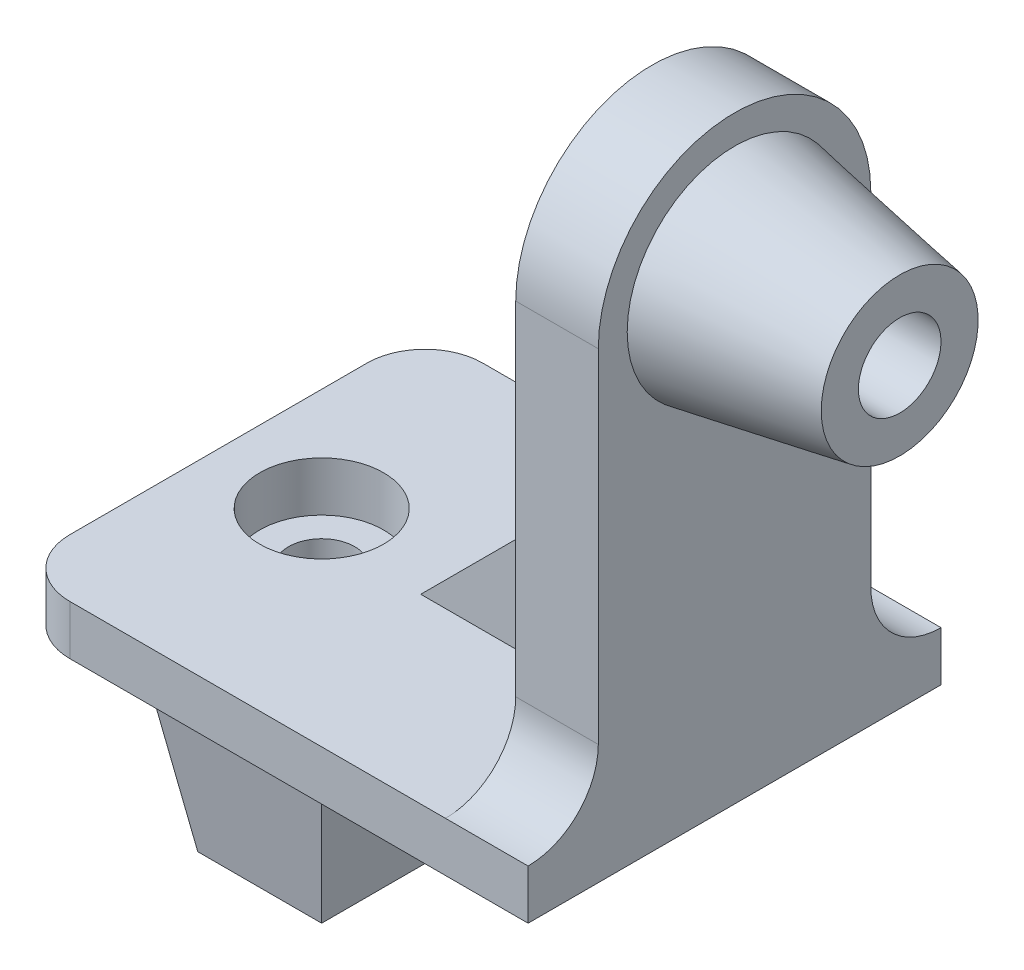
ISO-10303-21;
HEADER;
FILE_DESCRIPTION(('STEP AP214'),'2;1');
FILE_NAME('part.step','',(''),(''),'','','');
FILE_SCHEMA(('AUTOMOTIVE_DESIGN { 1 0 10303 214 1 1 1 1 }'));
ENDSEC;
DATA;
#1=APPLICATION_CONTEXT('core data for automotive mechanical design processes');
#2=APPLICATION_PROTOCOL_DEFINITION('international standard','automotive_design',2000,#1);
#3=PRODUCT_CONTEXT('',#1,'mechanical');
#4=PRODUCT('Part','Part','',(#3));
#5=PRODUCT_RELATED_PRODUCT_CATEGORY('part','',(#4));
#6=PRODUCT_DEFINITION_FORMATION('','',#4);
#7=PRODUCT_DEFINITION_CONTEXT('part definition',#1,'design');
#8=PRODUCT_DEFINITION('design','',#6,#7);
#9=PRODUCT_DEFINITION_SHAPE('','',#8);
#10=(LENGTH_UNIT() NAMED_UNIT(*) SI_UNIT(.MILLI.,.METRE.));
#11=(NAMED_UNIT(*) PLANE_ANGLE_UNIT() SI_UNIT($,.RADIAN.));
#12=(NAMED_UNIT(*) SI_UNIT($,.STERADIAN.) SOLID_ANGLE_UNIT());
#13=UNCERTAINTY_MEASURE_WITH_UNIT(LENGTH_MEASURE(1.E-05),#10,'distance_accuracy_value','');
#14=(GEOMETRIC_REPRESENTATION_CONTEXT(3) GLOBAL_UNCERTAINTY_ASSIGNED_CONTEXT((#13)) GLOBAL_UNIT_ASSIGNED_CONTEXT((#10,
#11,#12)) REPRESENTATION_CONTEXT('',''));
#15=CARTESIAN_POINT('',(0.,0.,0.));
#16=DIRECTION('',(0.,0.,1.));
#17=DIRECTION('',(1.,0.,0.));
#18=AXIS2_PLACEMENT_3D('',#15,#16,#17);
#19=CARTESIAN_POINT('',(-48.5,0.,-36.));
#20=DIRECTION('',(0.,-1.,0.));
#21=DIRECTION('',(0.,0.,-1.));
#22=AXIS2_PLACEMENT_3D('',#19,#20,#21);
#23=PLANE('',#22);
#24=DIRECTION('',(0.,0.,1.));
#25=VECTOR('',#24,1.);
#26=CARTESIAN_POINT('',(-12.5,0.,-25.));
#27=LINE('',#26,#25);
#28=CARTESIAN_POINT('',(-12.5,0.,-25.));
#29=VERTEX_POINT('',#28);
#30=CARTESIAN_POINT('',(-12.5,0.,25.));
#31=VERTEX_POINT('',#30);
#32=EDGE_CURVE('E178',#29,#31,#27,.T.);
#33=ORIENTED_EDGE('',*,*,#32,.F.);
#34=DIRECTION('',(1.,0.,0.));
#35=VECTOR('',#34,1.);
#36=CARTESIAN_POINT('',(-62.5,0.,-25.));
#37=LINE('',#36,#35);
#38=CARTESIAN_POINT('',(-62.5,0.,-25.));
#39=VERTEX_POINT('',#38);
#40=EDGE_CURVE('E257',#39,#29,#37,.T.);
#41=ORIENTED_EDGE('',*,*,#40,.F.);
#42=DIRECTION('',(0.,0.,1.));
#43=VECTOR('',#42,1.);
#44=CARTESIAN_POINT('',(-62.5,0.,36.));
#45=LINE('',#44,#43);
#46=CARTESIAN_POINT('',(-62.5,0.,-36.));
#47=VERTEX_POINT('',#46);
#48=EDGE_CURVE('E339',#47,#39,#45,.T.);
#49=ORIENTED_EDGE('',*,*,#48,.F.);
#50=CARTESIAN_POINT('',(-48.5,0.,-36.));
#51=DIRECTION('',(0.,1.,0.));
#52=DIRECTION('',(0.,0.,-1.));
#53=AXIS2_PLACEMENT_3D('',#50,#51,#52);
#54=CIRCLE('',#53,14.);
#55=CARTESIAN_POINT('',(-48.5,0.,-50.));
#56=VERTEX_POINT('',#55);
#57=EDGE_CURVE('E327',#56,#47,#54,.T.);
#58=ORIENTED_EDGE('',*,*,#57,.F.);
#59=DIRECTION('',(-1.,0.,0.));
#60=VECTOR('',#59,1.);
#61=CARTESIAN_POINT('',(-48.5,0.,-50.));
#62=LINE('',#61,#60);
#63=CARTESIAN_POINT('',(62.5,0.,-50.));
#64=VERTEX_POINT('',#63);
#65=EDGE_CURVE('E326',#64,#56,#62,.T.);
#66=ORIENTED_EDGE('',*,*,#65,.F.);
#67=DIRECTION('',(0.,0.,-1.));
#68=VECTOR('',#67,1.);
#69=CARTESIAN_POINT('',(62.5,0.,50.));
#70=LINE('',#69,#68);
#71=CARTESIAN_POINT('',(62.5,0.,50.));
#72=VERTEX_POINT('',#71);
#73=EDGE_CURVE('E307',#72,#64,#70,.T.);
#74=ORIENTED_EDGE('',*,*,#73,.F.);
#75=DIRECTION('',(1.,0.,0.));
#76=VECTOR('',#75,1.);
#77=CARTESIAN_POINT('',(-48.5,0.,50.));
#78=LINE('',#77,#76);
#79=CARTESIAN_POINT('',(-48.5,0.,50.));
#80=VERTEX_POINT('',#79);
#81=EDGE_CURVE('E378',#80,#72,#78,.T.);
#82=ORIENTED_EDGE('',*,*,#81,.F.);
#83=CARTESIAN_POINT('',(-48.5,0.,36.));
#84=DIRECTION('',(0.,1.,0.));
#85=DIRECTION('',(0.,0.,-1.));
#86=AXIS2_PLACEMENT_3D('',#83,#84,#85);
#87=CIRCLE('',#86,14.);
#88=CARTESIAN_POINT('',(-62.5,0.,36.));
#89=VERTEX_POINT('',#88);
#90=EDGE_CURVE('E334',#89,#80,#87,.T.);
#91=ORIENTED_EDGE('',*,*,#90,.F.);
#92=CARTESIAN_POINT('',(-62.5,0.,25.));
#93=VERTEX_POINT('',#92);
#94=EDGE_CURVE('E329',#93,#89,#45,.T.);
#95=ORIENTED_EDGE('',*,*,#94,.F.);
#96=DIRECTION('',(-1.,0.,0.));
#97=VECTOR('',#96,1.);
#98=CARTESIAN_POINT('',(-62.5,0.,25.));
#99=LINE('',#98,#97);
#100=EDGE_CURVE('E766',#31,#93,#99,.T.);
#101=ORIENTED_EDGE('',*,*,#100,.F.);
#102=EDGE_LOOP('',(#33,#41,#49,#58,#66,#74,#82,#91,#95,#101));
#103=FACE_BOUND('',#102,.T.);
#104=ADVANCED_FACE('F47',(#103),#23,.T.);
#105=CARTESIAN_POINT('',(62.5,12.,50.));
#106=DIRECTION('',(-1.,0.,0.));
#107=DIRECTION('',(0.,0.,1.));
#108=AXIS2_PLACEMENT_3D('',#105,#106,#107);
#109=PLANE('',#108);
#110=ORIENTED_EDGE('',*,*,#73,.T.);
#111=DIRECTION('',(0.,-1.,0.));
#112=VECTOR('',#111,1.);
#113=CARTESIAN_POINT('',(62.5,12.,-50.));
#114=LINE('',#113,#112);
#115=CARTESIAN_POINT('',(62.5,12.,-50.));
#116=VERTEX_POINT('',#115);
#117=EDGE_CURVE('E362',#116,#64,#114,.T.);
#118=ORIENTED_EDGE('',*,*,#117,.F.);
#119=CARTESIAN_POINT('',(62.5,29.,-50.));
#120=DIRECTION('',(-1.,0.,0.));
#121=DIRECTION('',(0.,0.,1.));
#122=AXIS2_PLACEMENT_3D('',#119,#120,#121);
#123=CIRCLE('',#122,17.);
#124=CARTESIAN_POINT('',(62.5,29.,-33.));
#125=VERTEX_POINT('',#124);
#126=EDGE_CURVE('E351',#116,#125,#123,.T.);
#127=ORIENTED_EDGE('',*,*,#126,.T.);
#128=DIRECTION('',(0.,1.,0.));
#129=VECTOR('',#128,1.);
#130=CARTESIAN_POINT('',(62.5,112.,-33.));
#131=LINE('',#130,#129);
#132=CARTESIAN_POINT('',(62.5,112.,-33.));
#133=VERTEX_POINT('',#132);
#134=EDGE_CURVE('E284',#125,#133,#131,.T.);
#135=ORIENTED_EDGE('',*,*,#134,.T.);
#136=CARTESIAN_POINT('',(62.5,112.,0.));
#137=DIRECTION('',(1.,0.,0.));
#138=DIRECTION('',(0.,0.,1.));
#139=AXIS2_PLACEMENT_3D('',#136,#137,#138);
#140=CIRCLE('',#139,33.);
#141=CARTESIAN_POINT('',(62.5,112.,33.));
#142=VERTEX_POINT('',#141);
#143=EDGE_CURVE('E299',#133,#142,#140,.T.);
#144=ORIENTED_EDGE('',*,*,#143,.T.);
#145=DIRECTION('',(0.,-1.,0.));
#146=VECTOR('',#145,1.);
#147=CARTESIAN_POINT('',(62.5,12.,33.));
#148=LINE('',#147,#146);
#149=CARTESIAN_POINT('',(62.5,29.,33.));
#150=VERTEX_POINT('',#149);
#151=EDGE_CURVE('E305',#142,#150,#148,.T.);
#152=ORIENTED_EDGE('',*,*,#151,.T.);
#153=CARTESIAN_POINT('',(62.5,29.,50.));
#154=DIRECTION('',(-1.,0.,0.));
#155=DIRECTION('',(0.,0.,1.));
#156=AXIS2_PLACEMENT_3D('',#153,#154,#155);
#157=CIRCLE('',#156,17.);
#158=CARTESIAN_POINT('',(62.5,12.,50.));
#159=VERTEX_POINT('',#158);
#160=EDGE_CURVE('E348',#150,#159,#157,.T.);
#161=ORIENTED_EDGE('',*,*,#160,.T.);
#162=DIRECTION('',(0.,-1.,0.));
#163=VECTOR('',#162,1.);
#164=CARTESIAN_POINT('',(62.5,12.,50.));
#165=LINE('',#164,#163);
#166=EDGE_CURVE('E322',#159,#72,#165,.T.);
#167=ORIENTED_EDGE('',*,*,#166,.T.);
#168=EDGE_LOOP('',(#110,#118,#127,#135,#144,#152,#161,#167));
#169=FACE_BOUND('',#168,.T.);
#170=CARTESIAN_POINT('',(62.5,112.,0.));
#171=DIRECTION('',(-1.,0.,0.));
#172=DIRECTION('',(0.,0.,1.));
#173=AXIS2_PLACEMENT_3D('',#170,#171,#172);
#174=CIRCLE('',#173,26.);
#175=CARTESIAN_POINT('',(62.5,112.,26.));
#176=VERTEX_POINT('',#175);
#177=EDGE_CURVE('E12',#176,#176,#174,.F.);
#178=ORIENTED_EDGE('',*,*,#177,.F.);
#179=EDGE_LOOP('',(#178));
#180=FACE_BOUND('',#179,.T.);
#181=ADVANCED_FACE('F399',(#169,#180),#109,.F.);
#182=CARTESIAN_POINT('',(-48.5,12.,-36.));
#183=DIRECTION('',(0.,-1.,0.));
#184=DIRECTION('',(0.,0.,-1.));
#185=AXIS2_PLACEMENT_3D('',#182,#183,#184);
#186=PLANE('',#185);
#187=CARTESIAN_POINT('',(-37.5,12.,0.));
#188=DIRECTION('',(0.,1.,0.));
#189=DIRECTION('',(0.,0.,1.));
#190=AXIS2_PLACEMENT_3D('',#187,#188,#189);
#191=CIRCLE('',#190,15.);
#192=CARTESIAN_POINT('',(-37.5,12.,15.));
#193=VERTEX_POINT('',#192);
#194=EDGE_CURVE('E702',#193,#193,#191,.T.);
#195=ORIENTED_EDGE('',*,*,#194,.F.);
#196=EDGE_LOOP('',(#195));
#197=FACE_BOUND('',#196,.T.);
#198=DIRECTION('',(0.,0.,-1.));
#199=VECTOR('',#198,1.);
#200=CARTESIAN_POINT('',(42.5,12.,-33.));
#201=LINE('',#200,#199);
#202=CARTESIAN_POINT('',(42.5,12.,50.));
#203=VERTEX_POINT('',#202);
#204=CARTESIAN_POINT('',(42.5,12.,6.));
#205=VERTEX_POINT('',#204);
#206=EDGE_CURVE('E281',#203,#205,#201,.T.);
#207=ORIENTED_EDGE('',*,*,#206,.T.);
#208=DIRECTION('',(-1.,0.,0.));
#209=VECTOR('',#208,1.);
#210=CARTESIAN_POINT('',(-48.5,12.,6.));
#211=LINE('',#210,#209);
#212=CARTESIAN_POINT('',(-7.49999999999999,12.,6.));
#213=VERTEX_POINT('',#212);
#214=EDGE_CURVE('E279',#205,#213,#211,.T.);
#215=ORIENTED_EDGE('',*,*,#214,.T.);
#216=DIRECTION('',(0.,0.,1.));
#217=VECTOR('',#216,1.);
#218=CARTESIAN_POINT('',(-7.49999999999999,12.,-36.));
#219=LINE('',#218,#217);
#220=CARTESIAN_POINT('',(-7.49999999999999,12.,-6.));
#221=VERTEX_POINT('',#220);
#222=EDGE_CURVE('E282',#213,#221,#219,.F.);
#223=ORIENTED_EDGE('',*,*,#222,.T.);
#224=DIRECTION('',(-1.,0.,0.));
#225=VECTOR('',#224,1.);
#226=CARTESIAN_POINT('',(-48.5,12.,-6.));
#227=LINE('',#226,#225);
#228=CARTESIAN_POINT('',(42.5,12.,-6.));
#229=VERTEX_POINT('',#228);
#230=EDGE_CURVE('E274',#229,#221,#227,.T.);
#231=ORIENTED_EDGE('',*,*,#230,.F.);
#232=CARTESIAN_POINT('',(42.5,12.,-50.));
#233=VERTEX_POINT('',#232);
#234=EDGE_CURVE('E286',#229,#233,#201,.T.);
#235=ORIENTED_EDGE('',*,*,#234,.T.);
#236=DIRECTION('',(-1.,0.,0.));
#237=VECTOR('',#236,1.);
#238=CARTESIAN_POINT('',(-48.5,12.,-50.));
#239=LINE('',#238,#237);
#240=CARTESIAN_POINT('',(-48.5,12.,-50.));
#241=VERTEX_POINT('',#240);
#242=EDGE_CURVE('E314',#233,#241,#239,.T.);
#243=ORIENTED_EDGE('',*,*,#242,.T.);
#244=CARTESIAN_POINT('',(-48.5,12.,-36.));
#245=DIRECTION('',(0.,1.,0.));
#246=DIRECTION('',(0.,0.,-1.));
#247=AXIS2_PLACEMENT_3D('',#244,#245,#246);
#248=CIRCLE('',#247,14.);
#249=CARTESIAN_POINT('',(-62.5,12.,-36.));
#250=VERTEX_POINT('',#249);
#251=EDGE_CURVE('E311',#241,#250,#248,.T.);
#252=ORIENTED_EDGE('',*,*,#251,.T.);
#253=DIRECTION('',(0.,0.,1.));
#254=VECTOR('',#253,1.);
#255=CARTESIAN_POINT('',(-62.5,12.,36.));
#256=LINE('',#255,#254);
#257=CARTESIAN_POINT('',(-62.5,12.,36.));
#258=VERTEX_POINT('',#257);
#259=EDGE_CURVE('E316',#250,#258,#256,.T.);
#260=ORIENTED_EDGE('',*,*,#259,.T.);
#261=CARTESIAN_POINT('',(-48.5,12.,36.));
#262=DIRECTION('',(0.,1.,0.));
#263=DIRECTION('',(0.,0.,-1.));
#264=AXIS2_PLACEMENT_3D('',#261,#262,#263);
#265=CIRCLE('',#264,14.);
#266=CARTESIAN_POINT('',(-48.5,12.,50.));
#267=VERTEX_POINT('',#266);
#268=EDGE_CURVE('E318',#258,#267,#265,.T.);
#269=ORIENTED_EDGE('',*,*,#268,.T.);
#270=DIRECTION('',(1.,0.,0.));
#271=VECTOR('',#270,1.);
#272=CARTESIAN_POINT('',(-48.5,12.,50.));
#273=LINE('',#272,#271);
#274=EDGE_CURVE('E321',#267,#203,#273,.T.);
#275=ORIENTED_EDGE('',*,*,#274,.T.);
#276=EDGE_LOOP('',(#207,#215,#223,#231,#235,#243,#252,#260,#269,#275));
#277=FACE_BOUND('',#276,.T.);
#278=ADVANCED_FACE('F429',(#197,#277),#186,.F.);
#279=CARTESIAN_POINT('',(-48.5,12.,-50.));
#280=DIRECTION('',(0.,0.,1.));
#281=DIRECTION('',(1.,0.,0.));
#282=AXIS2_PLACEMENT_3D('',#279,#280,#281);
#283=PLANE('',#282);
#284=ORIENTED_EDGE('',*,*,#65,.T.);
#285=DIRECTION('',(0.,-1.,0.));
#286=VECTOR('',#285,1.);
#287=CARTESIAN_POINT('',(-48.5,12.,-50.));
#288=LINE('',#287,#286);
#289=EDGE_CURVE('E364',#241,#56,#288,.T.);
#290=ORIENTED_EDGE('',*,*,#289,.F.);
#291=ORIENTED_EDGE('',*,*,#242,.F.);
#292=EDGE_CURVE('E309',#116,#233,#239,.T.);
#293=ORIENTED_EDGE('',*,*,#292,.F.);
#294=ORIENTED_EDGE('',*,*,#117,.T.);
#295=EDGE_LOOP('',(#284,#290,#291,#293,#294));
#296=FACE_BOUND('',#295,.T.);
#297=ADVANCED_FACE('F426',(#296),#283,.F.);
#298=CARTESIAN_POINT('',(-48.5,12.,-36.));
#299=DIRECTION('',(0.,-1.,0.));
#300=DIRECTION('',(0.,0.,-1.));
#301=AXIS2_PLACEMENT_3D('',#298,#299,#300);
#302=CYLINDRICAL_SURFACE('',#301,14.);
#303=ORIENTED_EDGE('',*,*,#57,.T.);
#304=DIRECTION('',(0.,-1.,0.));
#305=VECTOR('',#304,1.);
#306=CARTESIAN_POINT('',(-62.5,12.,-36.));
#307=LINE('',#306,#305);
#308=EDGE_CURVE('E366',#250,#47,#307,.T.);
#309=ORIENTED_EDGE('',*,*,#308,.F.);
#310=ORIENTED_EDGE('',*,*,#251,.F.);
#311=ORIENTED_EDGE('',*,*,#289,.T.);
#312=EDGE_LOOP('',(#303,#309,#310,#311));
#313=FACE_BOUND('',#312,.T.);
#314=ADVANCED_FACE('F470',(#313),#302,.T.);
#315=CARTESIAN_POINT('',(-62.5,12.,36.));
#316=DIRECTION('',(1.,0.,0.));
#317=DIRECTION('',(0.,0.,-1.));
#318=AXIS2_PLACEMENT_3D('',#315,#316,#317);
#319=PLANE('',#318);
#320=ORIENTED_EDGE('',*,*,#48,.T.);
#321=DIRECTION('',(0.,0.,-1.));
#322=VECTOR('',#321,1.);
#323=CARTESIAN_POINT('',(-62.5,0.,-25.));
#324=LINE('',#323,#322);
#325=EDGE_CURVE('E759',#93,#39,#324,.T.);
#326=ORIENTED_EDGE('',*,*,#325,.F.);
#327=ORIENTED_EDGE('',*,*,#94,.T.);
#328=DIRECTION('',(0.,-1.,0.));
#329=VECTOR('',#328,1.);
#330=CARTESIAN_POINT('',(-62.5,12.,36.));
#331=LINE('',#330,#329);
#332=EDGE_CURVE('E371',#258,#89,#331,.T.);
#333=ORIENTED_EDGE('',*,*,#332,.F.);
#334=ORIENTED_EDGE('',*,*,#259,.F.);
#335=ORIENTED_EDGE('',*,*,#308,.T.);
#336=EDGE_LOOP('',(#320,#326,#327,#333,#334,#335));
#337=FACE_BOUND('',#336,.T.);
#338=ADVANCED_FACE('F461',(#337),#319,.F.);
#339=CARTESIAN_POINT('',(-48.5,12.,36.));
#340=DIRECTION('',(0.,-1.,0.));
#341=DIRECTION('',(0.,0.,-1.));
#342=AXIS2_PLACEMENT_3D('',#339,#340,#341);
#343=CYLINDRICAL_SURFACE('',#342,14.);
#344=ORIENTED_EDGE('',*,*,#90,.T.);
#345=DIRECTION('',(0.,-1.,0.));
#346=VECTOR('',#345,1.);
#347=CARTESIAN_POINT('',(-48.5,12.,50.));
#348=LINE('',#347,#346);
#349=EDGE_CURVE('E372',#267,#80,#348,.T.);
#350=ORIENTED_EDGE('',*,*,#349,.F.);
#351=ORIENTED_EDGE('',*,*,#268,.F.);
#352=ORIENTED_EDGE('',*,*,#332,.T.);
#353=EDGE_LOOP('',(#344,#350,#351,#352));
#354=FACE_BOUND('',#353,.T.);
#355=ADVANCED_FACE('F384',(#354),#343,.T.);
#356=CARTESIAN_POINT('',(-48.5,12.,50.));
#357=DIRECTION('',(0.,0.,-1.));
#358=DIRECTION('',(-1.,0.,0.));
#359=AXIS2_PLACEMENT_3D('',#356,#357,#358);
#360=PLANE('',#359);
#361=ORIENTED_EDGE('',*,*,#81,.T.);
#362=ORIENTED_EDGE('',*,*,#166,.F.);
#363=EDGE_CURVE('E319',#203,#159,#273,.T.);
#364=ORIENTED_EDGE('',*,*,#363,.F.);
#365=ORIENTED_EDGE('',*,*,#274,.F.);
#366=ORIENTED_EDGE('',*,*,#349,.T.);
#367=EDGE_LOOP('',(#361,#362,#364,#365,#366));
#368=FACE_BOUND('',#367,.T.);
#369=ADVANCED_FACE('F392',(#368),#360,.F.);
#370=CARTESIAN_POINT('',(42.5,12.,33.));
#371=DIRECTION('',(0.,0.,1.));
#372=DIRECTION('',(0.,-1.,0.));
#373=AXIS2_PLACEMENT_3D('',#370,#371,#372);
#374=PLANE('',#373);
#375=DIRECTION('',(0.,-1.,0.));
#376=VECTOR('',#375,1.);
#377=CARTESIAN_POINT('',(42.5,12.,33.));
#378=LINE('',#377,#376);
#379=CARTESIAN_POINT('',(42.5,112.,33.));
#380=VERTEX_POINT('',#379);
#381=CARTESIAN_POINT('',(42.5,29.,33.));
#382=VERTEX_POINT('',#381);
#383=EDGE_CURVE('E294',#380,#382,#378,.T.);
#384=ORIENTED_EDGE('',*,*,#383,.T.);
#385=DIRECTION('',(1.,0.,0.));
#386=VECTOR('',#385,1.);
#387=CARTESIAN_POINT('',(42.5,29.,33.));
#388=LINE('',#387,#386);
#389=EDGE_CURVE('E360',#382,#150,#388,.T.);
#390=ORIENTED_EDGE('',*,*,#389,.T.);
#391=ORIENTED_EDGE('',*,*,#151,.F.);
#392=DIRECTION('',(1.,0.,0.));
#393=VECTOR('',#392,1.);
#394=CARTESIAN_POINT('',(42.5,112.,33.));
#395=LINE('',#394,#393);
#396=EDGE_CURVE('E303',#380,#142,#395,.T.);
#397=ORIENTED_EDGE('',*,*,#396,.F.);
#398=EDGE_LOOP('',(#384,#390,#391,#397));
#399=FACE_BOUND('',#398,.T.);
#400=ADVANCED_FACE('F406',(#399),#374,.T.);
#401=CARTESIAN_POINT('',(42.5,112.,0.));
#402=DIRECTION('',(1.,0.,0.));
#403=DIRECTION('',(0.,0.,-1.));
#404=AXIS2_PLACEMENT_3D('',#401,#402,#403);
#405=CYLINDRICAL_SURFACE('',#404,33.);
#406=ORIENTED_EDGE('',*,*,#143,.F.);
#407=DIRECTION('',(1.,0.,0.));
#408=VECTOR('',#407,1.);
#409=CARTESIAN_POINT('',(42.5,112.,-33.));
#410=LINE('',#409,#408);
#411=CARTESIAN_POINT('',(42.5,112.,-33.));
#412=VERTEX_POINT('',#411);
#413=EDGE_CURVE('E300',#412,#133,#410,.T.);
#414=ORIENTED_EDGE('',*,*,#413,.F.);
#415=CARTESIAN_POINT('',(42.5,112.,0.));
#416=DIRECTION('',(1.,0.,0.));
#417=DIRECTION('',(0.,0.,1.));
#418=AXIS2_PLACEMENT_3D('',#415,#416,#417);
#419=CIRCLE('',#418,33.);
#420=EDGE_CURVE('E292',#412,#380,#419,.T.);
#421=ORIENTED_EDGE('',*,*,#420,.T.);
#422=ORIENTED_EDGE('',*,*,#396,.T.);
#423=EDGE_LOOP('',(#406,#414,#421,#422));
#424=FACE_BOUND('',#423,.T.);
#425=ADVANCED_FACE('F413',(#424),#405,.T.);
#426=CARTESIAN_POINT('',(42.5,112.,-33.));
#427=DIRECTION('',(0.,0.,-1.));
#428=DIRECTION('',(0.,1.,0.));
#429=AXIS2_PLACEMENT_3D('',#426,#427,#428);
#430=PLANE('',#429);
#431=ORIENTED_EDGE('',*,*,#134,.F.);
#432=DIRECTION('',(1.,0.,0.));
#433=VECTOR('',#432,1.);
#434=CARTESIAN_POINT('',(42.5,29.,-33.));
#435=LINE('',#434,#433);
#436=CARTESIAN_POINT('',(42.5,29.,-33.));
#437=VERTEX_POINT('',#436);
#438=EDGE_CURVE('E358',#125,#437,#435,.F.);
#439=ORIENTED_EDGE('',*,*,#438,.T.);
#440=DIRECTION('',(0.,1.,0.));
#441=VECTOR('',#440,1.);
#442=CARTESIAN_POINT('',(42.5,112.,-33.));
#443=LINE('',#442,#441);
#444=EDGE_CURVE('E289',#437,#412,#443,.T.);
#445=ORIENTED_EDGE('',*,*,#444,.T.);
#446=ORIENTED_EDGE('',*,*,#413,.T.);
#447=EDGE_LOOP('',(#431,#439,#445,#446));
#448=FACE_BOUND('',#447,.T.);
#449=ADVANCED_FACE('F479',(#448),#430,.T.);
#450=CARTESIAN_POINT('',(42.5,112.,0.));
#451=DIRECTION('',(-1.,0.,0.));
#452=DIRECTION('',(0.,0.,1.));
#453=AXIS2_PLACEMENT_3D('',#450,#451,#452);
#454=PLANE('',#453);
#455=CARTESIAN_POINT('',(42.5,112.,0.));
#456=DIRECTION('',(-1.,0.,0.));
#457=DIRECTION('',(0.,0.,1.));
#458=AXIS2_PLACEMENT_3D('',#455,#456,#457);
#459=CIRCLE('',#458,15.);
#460=CARTESIAN_POINT('',(42.5,112.,15.));
#461=VERTEX_POINT('',#460);
#462=EDGE_CURVE('E259',#461,#461,#459,.T.);
#463=ORIENTED_EDGE('',*,*,#462,.F.);
#464=EDGE_LOOP('',(#463));
#465=FACE_BOUND('',#464,.T.);
#466=DIRECTION('',(0.,1.,0.));
#467=VECTOR('',#466,1.);
#468=CARTESIAN_POINT('',(42.5,112.,6.));
#469=LINE('',#468,#467);
#470=CARTESIAN_POINT('',(42.5,62.,6.));
#471=VERTEX_POINT('',#470);
#472=EDGE_CURVE('E59',#205,#471,#469,.T.);
#473=ORIENTED_EDGE('',*,*,#472,.F.);
#474=ORIENTED_EDGE('',*,*,#206,.F.);
#475=CARTESIAN_POINT('',(42.5,29.,50.));
#476=DIRECTION('',(-1.,0.,0.));
#477=DIRECTION('',(0.,0.,1.));
#478=AXIS2_PLACEMENT_3D('',#475,#476,#477);
#479=CIRCLE('',#478,17.);
#480=EDGE_CURVE('E346',#203,#382,#479,.F.);
#481=ORIENTED_EDGE('',*,*,#480,.T.);
#482=ORIENTED_EDGE('',*,*,#383,.F.);
#483=ORIENTED_EDGE('',*,*,#420,.F.);
#484=ORIENTED_EDGE('',*,*,#444,.F.);
#485=CARTESIAN_POINT('',(42.5,29.,-50.));
#486=DIRECTION('',(-1.,0.,0.));
#487=DIRECTION('',(0.,0.,1.));
#488=AXIS2_PLACEMENT_3D('',#485,#486,#487);
#489=CIRCLE('',#488,17.);
#490=EDGE_CURVE('E355',#437,#233,#489,.F.);
#491=ORIENTED_EDGE('',*,*,#490,.T.);
#492=ORIENTED_EDGE('',*,*,#234,.F.);
#493=DIRECTION('',(0.,1.,0.));
#494=VECTOR('',#493,1.);
#495=CARTESIAN_POINT('',(42.5,112.,-6.));
#496=LINE('',#495,#494);
#497=CARTESIAN_POINT('',(42.5,62.,-6.));
#498=VERTEX_POINT('',#497);
#499=EDGE_CURVE('E343',#229,#498,#496,.T.);
#500=ORIENTED_EDGE('',*,*,#499,.T.);
#501=DIRECTION('',(0.,0.,1.));
#502=VECTOR('',#501,1.);
#503=CARTESIAN_POINT('',(42.5,62.,0.));
#504=LINE('',#503,#502);
#505=EDGE_CURVE('E344',#471,#498,#504,.F.);
#506=ORIENTED_EDGE('',*,*,#505,.F.);
#507=EDGE_LOOP('',(#473,#474,#481,#482,#483,#484,#491,#492,#500,#506));
#508=FACE_BOUND('',#507,.T.);
#509=ADVANCED_FACE('F410',(#465,#508),#454,.T.);
#510=CARTESIAN_POINT('',(-48.5,29.,-50.));
#511=DIRECTION('',(1.,0.,0.));
#512=DIRECTION('',(0.,0.,-1.));
#513=AXIS2_PLACEMENT_3D('',#510,#511,#512);
#514=CYLINDRICAL_SURFACE('',#513,17.);
#515=ORIENTED_EDGE('',*,*,#490,.F.);
#516=ORIENTED_EDGE('',*,*,#438,.F.);
#517=ORIENTED_EDGE('',*,*,#126,.F.);
#518=ORIENTED_EDGE('',*,*,#292,.T.);
#519=EDGE_LOOP('',(#515,#516,#517,#518));
#520=FACE_BOUND('',#519,.T.);
#521=ADVANCED_FACE('F421',(#520),#514,.F.);
#522=CARTESIAN_POINT('',(42.5,29.,50.));
#523=DIRECTION('',(1.,0.,0.));
#524=DIRECTION('',(0.,0.,-1.));
#525=AXIS2_PLACEMENT_3D('',#522,#523,#524);
#526=CYLINDRICAL_SURFACE('',#525,17.);
#527=ORIENTED_EDGE('',*,*,#480,.F.);
#528=ORIENTED_EDGE('',*,*,#363,.T.);
#529=ORIENTED_EDGE('',*,*,#160,.F.);
#530=ORIENTED_EDGE('',*,*,#389,.F.);
#531=EDGE_LOOP('',(#527,#528,#529,#530));
#532=FACE_BOUND('',#531,.T.);
#533=ADVANCED_FACE('F51',(#532),#526,.F.);
#534=CARTESIAN_POINT('',(-7.49999999999999,12.,0.));
#535=DIRECTION('',(0.707106781186548,-0.707106781186548,0.));
#536=DIRECTION('',(0.707106781186547,0.707106781186547,0.));
#537=AXIS2_PLACEMENT_3D('',#534,#535,#536);
#538=PLANE('',#537);
#539=ORIENTED_EDGE('',*,*,#222,.F.);
#540=DIRECTION('',(0.707106781186547,0.707106781186547,0.));
#541=VECTOR('',#540,1.);
#542=CARTESIAN_POINT('',(-7.49999999999999,12.,6.));
#543=LINE('',#542,#541);
#544=EDGE_CURVE('E275',#213,#471,#543,.T.);
#545=ORIENTED_EDGE('',*,*,#544,.T.);
#546=ORIENTED_EDGE('',*,*,#505,.T.);
#547=DIRECTION('',(0.707106781186547,0.707106781186547,0.));
#548=VECTOR('',#547,1.);
#549=CARTESIAN_POINT('',(-7.49999999999999,12.,-6.));
#550=LINE('',#549,#548);
#551=EDGE_CURVE('E74',#221,#498,#550,.T.);
#552=ORIENTED_EDGE('',*,*,#551,.F.);
#553=EDGE_LOOP('',(#539,#545,#546,#552));
#554=FACE_BOUND('',#553,.T.);
#555=ADVANCED_FACE('F436',(#554),#538,.F.);
#556=CARTESIAN_POINT('',(0.,72.5,6.));
#557=DIRECTION('',(0.,0.,1.));
#558=DIRECTION('',(1.,0.,0.));
#559=AXIS2_PLACEMENT_3D('',#556,#557,#558);
#560=PLANE('',#559);
#561=ORIENTED_EDGE('',*,*,#214,.F.);
#562=ORIENTED_EDGE('',*,*,#472,.T.);
#563=ORIENTED_EDGE('',*,*,#544,.F.);
#564=EDGE_LOOP('',(#561,#562,#563));
#565=FACE_BOUND('',#564,.T.);
#566=ADVANCED_FACE('F438',(#565),#560,.T.);
#567=CARTESIAN_POINT('',(0.,72.5,-6.));
#568=DIRECTION('',(0.,0.,1.));
#569=DIRECTION('',(1.,0.,0.));
#570=AXIS2_PLACEMENT_3D('',#567,#568,#569);
#571=PLANE('',#570);
#572=ORIENTED_EDGE('',*,*,#499,.F.);
#573=ORIENTED_EDGE('',*,*,#230,.T.);
#574=ORIENTED_EDGE('',*,*,#551,.T.);
#575=EDGE_LOOP('',(#572,#573,#574));
#576=FACE_BOUND('',#575,.T.);
#577=ADVANCED_FACE('F432',(#576),#571,.F.);
#578=CARTESIAN_POINT('',(102.5,112.,0.));
#579=DIRECTION('',(-1.,0.,0.));
#580=DIRECTION('',(0.,0.,1.));
#581=AXIS2_PLACEMENT_3D('',#578,#579,#580);
#582=CONICAL_SURFACE('',#581,19.,0.173245666452365);
#583=ORIENTED_EDGE('',*,*,#177,.T.);
#584=EDGE_LOOP('',(#583));
#585=FACE_BOUND('',#584,.T.);
#586=CARTESIAN_POINT('',(102.5,112.,0.));
#587=DIRECTION('',(-1.,0.,0.));
#588=DIRECTION('',(0.,0.,1.));
#589=AXIS2_PLACEMENT_3D('',#586,#587,#588);
#590=CIRCLE('',#589,19.);
#591=CARTESIAN_POINT('',(102.5,112.,19.));
#592=VERTEX_POINT('',#591);
#593=EDGE_CURVE('E267',#592,#592,#590,.T.);
#594=ORIENTED_EDGE('',*,*,#593,.T.);
#595=EDGE_LOOP('',(#594));
#596=FACE_BOUND('',#595,.T.);
#597=ADVANCED_FACE('F447',(#585,#596),#582,.T.);
#598=CARTESIAN_POINT('',(102.5,131.,0.));
#599=DIRECTION('',(-1.,0.,0.));
#600=DIRECTION('',(0.,0.,1.));
#601=AXIS2_PLACEMENT_3D('',#598,#599,#600);
#602=PLANE('',#601);
#603=ORIENTED_EDGE('',*,*,#593,.F.);
#604=EDGE_LOOP('',(#603));
#605=FACE_BOUND('',#604,.T.);
#606=CARTESIAN_POINT('',(102.5,112.,0.));
#607=DIRECTION('',(-1.,0.,0.));
#608=DIRECTION('',(0.,0.,1.));
#609=AXIS2_PLACEMENT_3D('',#606,#607,#608);
#610=CIRCLE('',#609,9.99999999999999);
#611=CARTESIAN_POINT('',(102.5,112.,9.99999999999999));
#612=VERTEX_POINT('',#611);
#613=EDGE_CURVE('E262',#612,#612,#610,.T.);
#614=ORIENTED_EDGE('',*,*,#613,.T.);
#615=EDGE_LOOP('',(#614));
#616=FACE_BOUND('',#615,.T.);
#617=ADVANCED_FACE('F563',(#605,#616),#602,.F.);
#618=CARTESIAN_POINT('',(62.5,112.,0.));
#619=DIRECTION('',(-1.,0.,0.));
#620=DIRECTION('',(0.,0.,1.));
#621=AXIS2_PLACEMENT_3D('',#618,#619,#620);
#622=CYLINDRICAL_SURFACE('',#621,9.99999999999999);
#623=ORIENTED_EDGE('',*,*,#613,.F.);
#624=EDGE_LOOP('',(#623));
#625=FACE_BOUND('',#624,.T.);
#626=CARTESIAN_POINT('',(54.5,112.,0.));
#627=DIRECTION('',(-1.,0.,0.));
#628=DIRECTION('',(0.,0.,1.));
#629=AXIS2_PLACEMENT_3D('',#626,#627,#628);
#630=CIRCLE('',#629,10.);
#631=CARTESIAN_POINT('',(54.5,112.,10.));
#632=VERTEX_POINT('',#631);
#633=EDGE_CURVE('E253',#632,#632,#630,.T.);
#634=ORIENTED_EDGE('',*,*,#633,.T.);
#635=EDGE_LOOP('',(#634));
#636=FACE_BOUND('',#635,.T.);
#637=ADVANCED_FACE('F573',(#625,#636),#622,.F.);
#638=CARTESIAN_POINT('',(54.5,112.,0.));
#639=DIRECTION('',(-1.,0.,0.));
#640=DIRECTION('',(0.,0.,1.));
#641=AXIS2_PLACEMENT_3D('',#638,#639,#640);
#642=CYLINDRICAL_SURFACE('',#641,15.);
#643=CARTESIAN_POINT('',(54.5,112.,0.));
#644=DIRECTION('',(-1.,0.,0.));
#645=DIRECTION('',(0.,0.,1.));
#646=AXIS2_PLACEMENT_3D('',#643,#644,#645);
#647=CIRCLE('',#646,15.);
#648=CARTESIAN_POINT('',(54.5,112.,15.));
#649=VERTEX_POINT('',#648);
#650=EDGE_CURVE('E261',#649,#649,#647,.T.);
#651=ORIENTED_EDGE('',*,*,#650,.F.);
#652=EDGE_LOOP('',(#651));
#653=FACE_BOUND('',#652,.T.);
#654=ORIENTED_EDGE('',*,*,#462,.T.);
#655=EDGE_LOOP('',(#654));
#656=FACE_BOUND('',#655,.T.);
#657=ADVANCED_FACE('F585',(#653,#656),#642,.F.);
#658=CARTESIAN_POINT('',(54.5,112.,0.));
#659=DIRECTION('',(-1.,0.,0.));
#660=DIRECTION('',(0.,0.,1.));
#661=AXIS2_PLACEMENT_3D('',#658,#659,#660);
#662=PLANE('',#661);
#663=ORIENTED_EDGE('',*,*,#633,.F.);
#664=EDGE_LOOP('',(#663));
#665=FACE_BOUND('',#664,.T.);
#666=ORIENTED_EDGE('',*,*,#650,.T.);
#667=EDGE_LOOP('',(#666));
#668=FACE_BOUND('',#667,.T.);
#669=ADVANCED_FACE('F225',(#665,#668),#662,.T.);
#670=CARTESIAN_POINT('',(0.,-60.,0.));
#671=DIRECTION('',(0.,1.,0.));
#672=DIRECTION('',(0.,0.,1.));
#673=AXIS2_PLACEMENT_3D('',#670,#671,#672);
#674=PLANE('',#673);
#675=CARTESIAN_POINT('',(-37.5,-60.,0.));
#676=DIRECTION('',(0.,1.,0.));
#677=DIRECTION('',(0.,0.,1.));
#678=AXIS2_PLACEMENT_3D('',#675,#676,#677);
#679=CIRCLE('',#678,8.00000000000001);
#680=CARTESIAN_POINT('',(-37.5,-60.,8.00000000000001));
#681=VERTEX_POINT('',#680);
#682=EDGE_CURVE('E52',#681,#681,#679,.T.);
#683=ORIENTED_EDGE('',*,*,#682,.T.);
#684=EDGE_LOOP('',(#683));
#685=FACE_BOUND('',#684,.T.);
#686=DIRECTION('',(0.,0.,-1.));
#687=VECTOR('',#686,1.);
#688=CARTESIAN_POINT('',(-52.5,-60.,15.));
#689=LINE('',#688,#687);
#690=CARTESIAN_POINT('',(-52.5,-60.,15.));
#691=VERTEX_POINT('',#690);
#692=CARTESIAN_POINT('',(-52.5,-60.,-15.));
#693=VERTEX_POINT('',#692);
#694=EDGE_CURVE('E247',#691,#693,#689,.T.);
#695=ORIENTED_EDGE('',*,*,#694,.T.);
#696=DIRECTION('',(1.,0.,0.));
#697=VECTOR('',#696,1.);
#698=CARTESIAN_POINT('',(-22.5,-60.,-15.));
#699=LINE('',#698,#697);
#700=CARTESIAN_POINT('',(-22.5,-60.,-15.));
#701=VERTEX_POINT('',#700);
#702=EDGE_CURVE('E203',#693,#701,#699,.T.);
#703=ORIENTED_EDGE('',*,*,#702,.T.);
#704=DIRECTION('',(0.,0.,1.));
#705=VECTOR('',#704,1.);
#706=CARTESIAN_POINT('',(-22.5,-60.,15.));
#707=LINE('',#706,#705);
#708=CARTESIAN_POINT('',(-22.5,-60.,15.));
#709=VERTEX_POINT('',#708);
#710=EDGE_CURVE('E177',#701,#709,#707,.T.);
#711=ORIENTED_EDGE('',*,*,#710,.T.);
#712=DIRECTION('',(-1.,0.,0.));
#713=VECTOR('',#712,1.);
#714=CARTESIAN_POINT('',(-22.5,-60.,15.));
#715=LINE('',#714,#713);
#716=EDGE_CURVE('E187',#709,#691,#715,.T.);
#717=ORIENTED_EDGE('',*,*,#716,.T.);
#718=EDGE_LOOP('',(#695,#703,#711,#717));
#719=FACE_BOUND('',#718,.T.);
#720=ADVANCED_FACE('F199',(#685,#719),#674,.F.);
#721=CARTESIAN_POINT('',(-60.8108108108108,-10.1351351351351,0.));
#722=DIRECTION('',(-0.986393923832144,-0.164398987305357,0.));
#723=DIRECTION('',(0.164398987305357,-0.986393923832144,0.));
#724=AXIS2_PLACEMENT_3D('',#721,#722,#723);
#725=PLANE('',#724);
#726=DIRECTION('',(-0.162221421130763,0.973328526784575,0.162221421130763));
#727=VECTOR('',#726,1.);
#728=CARTESIAN_POINT('',(-52.5,-60.,15.));
#729=LINE('',#728,#727);
#730=EDGE_CURVE('E186',#691,#93,#729,.T.);
#731=ORIENTED_EDGE('',*,*,#730,.T.);
#732=ORIENTED_EDGE('',*,*,#325,.T.);
#733=DIRECTION('',(-0.162221421130763,0.973328526784575,-0.162221421130763));
#734=VECTOR('',#733,1.);
#735=CARTESIAN_POINT('',(-52.5,-60.,-15.));
#736=LINE('',#735,#734);
#737=EDGE_CURVE('E181',#693,#39,#736,.T.);
#738=ORIENTED_EDGE('',*,*,#737,.F.);
#739=ORIENTED_EDGE('',*,*,#694,.F.);
#740=EDGE_LOOP('',(#731,#732,#738,#739));
#741=FACE_BOUND('',#740,.T.);
#742=ADVANCED_FACE('F222',(#741),#725,.T.);
#743=CARTESIAN_POINT('',(0.,-4.05405405405405,-24.3243243243243));
#744=DIRECTION('',(0.,-0.164398987305357,-0.986393923832144));
#745=DIRECTION('',(0.,0.986393923832144,-0.164398987305357));
#746=AXIS2_PLACEMENT_3D('',#743,#744,#745);
#747=PLANE('',#746);
#748=ORIENTED_EDGE('',*,*,#737,.T.);
#749=ORIENTED_EDGE('',*,*,#40,.T.);
#750=DIRECTION('',(0.162221421130763,0.973328526784575,-0.162221421130763));
#751=VECTOR('',#750,1.);
#752=CARTESIAN_POINT('',(-22.5,-60.,-15.));
#753=LINE('',#752,#751);
#754=EDGE_CURVE('E185',#701,#29,#753,.T.);
#755=ORIENTED_EDGE('',*,*,#754,.F.);
#756=ORIENTED_EDGE('',*,*,#702,.F.);
#757=EDGE_LOOP('',(#748,#749,#755,#756));
#758=FACE_BOUND('',#757,.T.);
#759=ADVANCED_FACE('F618',(#758),#747,.T.);
#760=CARTESIAN_POINT('',(0.,-4.05405405405406,24.3243243243243));
#761=DIRECTION('',(0.,-0.164398987305357,0.986393923832144));
#762=DIRECTION('',(0.,-0.986393923832144,-0.164398987305357));
#763=AXIS2_PLACEMENT_3D('',#760,#761,#762);
#764=PLANE('',#763);
#765=DIRECTION('',(0.162221421130763,0.973328526784575,0.162221421130763));
#766=VECTOR('',#765,1.);
#767=CARTESIAN_POINT('',(-22.5,-60.,15.));
#768=LINE('',#767,#766);
#769=EDGE_CURVE('E67',#709,#31,#768,.T.);
#770=ORIENTED_EDGE('',*,*,#769,.T.);
#771=ORIENTED_EDGE('',*,*,#100,.T.);
#772=ORIENTED_EDGE('',*,*,#730,.F.);
#773=ORIENTED_EDGE('',*,*,#716,.F.);
#774=EDGE_LOOP('',(#770,#771,#772,#773));
#775=FACE_BOUND('',#774,.T.);
#776=ADVANCED_FACE('F188',(#775),#764,.T.);
#777=CARTESIAN_POINT('',(-12.1621621621622,2.02702702702703,0.));
#778=DIRECTION('',(0.986393923832144,-0.164398987305357,0.));
#779=DIRECTION('',(0.164398987305357,0.986393923832144,0.));
#780=AXIS2_PLACEMENT_3D('',#777,#778,#779);
#781=PLANE('',#780);
#782=ORIENTED_EDGE('',*,*,#754,.T.);
#783=ORIENTED_EDGE('',*,*,#32,.T.);
#784=ORIENTED_EDGE('',*,*,#769,.F.);
#785=ORIENTED_EDGE('',*,*,#710,.F.);
#786=EDGE_LOOP('',(#782,#783,#784,#785));
#787=FACE_BOUND('',#786,.T.);
#788=ADVANCED_FACE('F174',(#787),#781,.T.);
#789=CARTESIAN_POINT('',(-37.5,12.,0.));
#790=DIRECTION('',(0.,1.,0.));
#791=DIRECTION('',(0.,0.,1.));
#792=AXIS2_PLACEMENT_3D('',#789,#790,#791);
#793=CYLINDRICAL_SURFACE('',#792,8.00000000000001);
#794=CARTESIAN_POINT('',(-37.5,0.,0.));
#795=DIRECTION('',(0.,1.,0.));
#796=DIRECTION('',(0.,0.,1.));
#797=AXIS2_PLACEMENT_3D('',#794,#795,#796);
#798=CIRCLE('',#797,8.00000000000001);
#799=CARTESIAN_POINT('',(-37.5,0.,8.00000000000002));
#800=VERTEX_POINT('',#799);
#801=EDGE_CURVE('E707',#800,#800,#798,.T.);
#802=ORIENTED_EDGE('',*,*,#801,.T.);
#803=EDGE_LOOP('',(#802));
#804=FACE_BOUND('',#803,.T.);
#805=ORIENTED_EDGE('',*,*,#682,.F.);
#806=EDGE_LOOP('',(#805));
#807=FACE_BOUND('',#806,.T.);
#808=ADVANCED_FACE('F221',(#804,#807),#793,.F.);
#809=CARTESIAN_POINT('',(-29.5,0.,0.));
#810=DIRECTION('',(0.,-1.,0.));
#811=DIRECTION('',(0.,0.,-1.));
#812=AXIS2_PLACEMENT_3D('',#809,#810,#811);
#813=PLANE('',#812);
#814=ORIENTED_EDGE('',*,*,#801,.F.);
#815=EDGE_LOOP('',(#814));
#816=FACE_BOUND('',#815,.T.);
#817=CARTESIAN_POINT('',(-37.5,0.,0.));
#818=DIRECTION('',(0.,1.,0.));
#819=DIRECTION('',(0.,0.,1.));
#820=AXIS2_PLACEMENT_3D('',#817,#818,#819);
#821=CIRCLE('',#820,15.);
#822=CARTESIAN_POINT('',(-37.5,0.,15.));
#823=VERTEX_POINT('',#822);
#824=EDGE_CURVE('E706',#823,#823,#821,.T.);
#825=ORIENTED_EDGE('',*,*,#824,.T.);
#826=EDGE_LOOP('',(#825));
#827=FACE_BOUND('',#826,.T.);
#828=ADVANCED_FACE('F647',(#816,#827),#813,.F.);
#829=CARTESIAN_POINT('',(-37.5,12.,0.));
#830=DIRECTION('',(0.,1.,0.));
#831=DIRECTION('',(0.,0.,1.));
#832=AXIS2_PLACEMENT_3D('',#829,#830,#831);
#833=CYLINDRICAL_SURFACE('',#832,15.);
#834=ORIENTED_EDGE('',*,*,#824,.F.);
#835=EDGE_LOOP('',(#834));
#836=FACE_BOUND('',#835,.T.);
#837=ORIENTED_EDGE('',*,*,#194,.T.);
#838=EDGE_LOOP('',(#837));
#839=FACE_BOUND('',#838,.T.);
#840=ADVANCED_FACE('F660',(#836,#839),#833,.F.);
#841=CLOSED_SHELL('',(#104,#181,#278,#297,#314,#338,#355,#369,#400,#425,#449,#509,#521,#533,
#555,#566,#577,#597,#617,#637,#657,#669,#720,#742,#759,#776,#788,#808,#828,#840));
#842=MANIFOLD_SOLID_BREP('B2',#841);
#843=ADVANCED_BREP_SHAPE_REPRESENTATION('',(#18,#842),#14);
#844=SHAPE_DEFINITION_REPRESENTATION(#9,#843);
ENDSEC;
END-ISO-10303-21;
